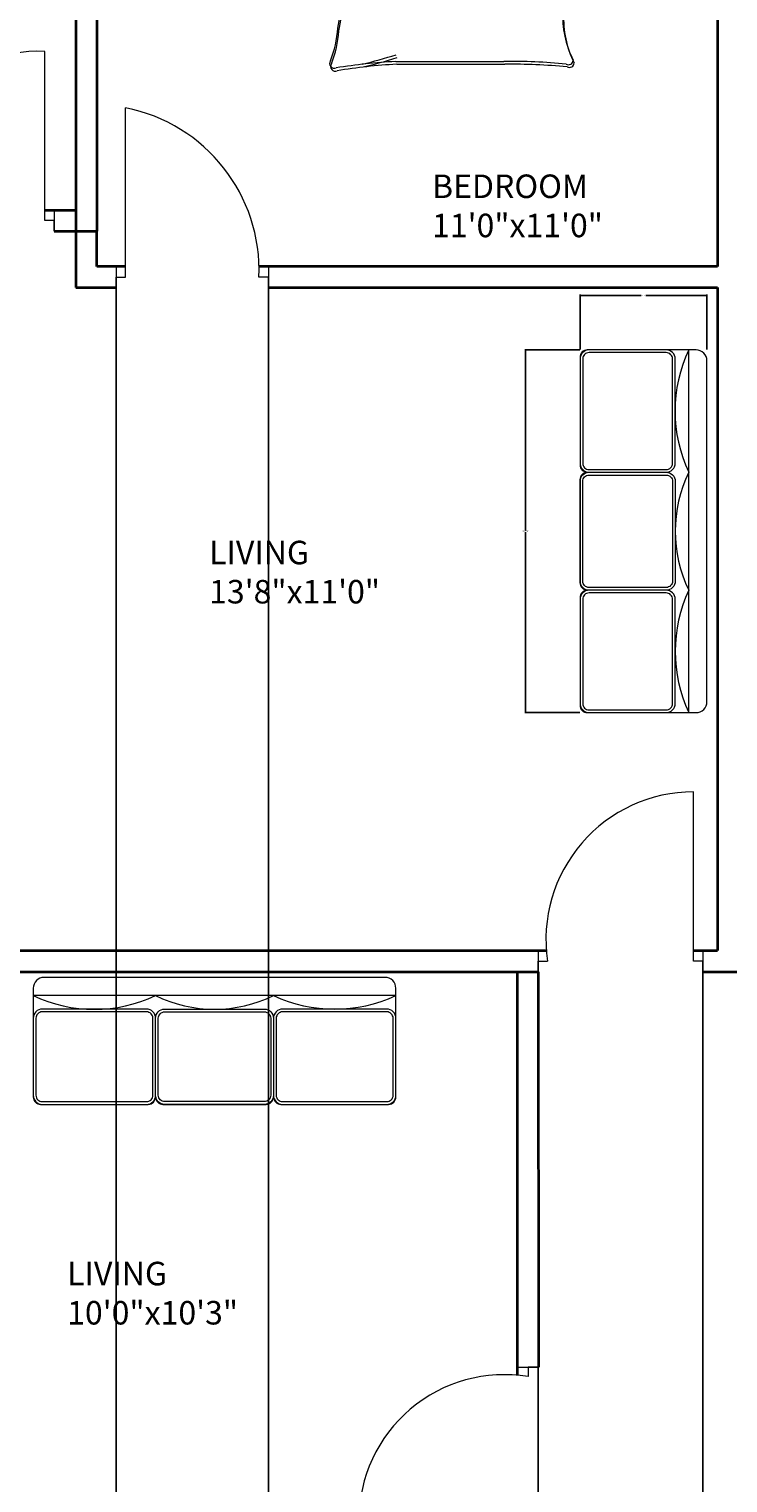
# Model space of a CAD drawing. Units: inches. Extents: x 2234 to 3001, y 1541 to 2386.
# Tile 6 of 12: x 2450 to 2599, y 1891 to 2201. Entities that reach past the tile are written whole.
import ezdxf

# ---------------------------------------------------------------- set-up
doc = ezdxf.new("R2010")
doc.units = ezdxf.units.IN
for name, color, linetype, lineweight in [('A-ANNO-DIMS', 2, 'Continuous', 18), ('A-AREA-IDEN', 7, 'Continuous', 18), ('A-DOOR', 3, 'Continuous', 18), ('A-FURN', 9, 'Continuous', 13), ('A-WALL', 7, 'Continuous', 35)]:
    doc.layers.add(name, color=color, linetype=linetype, lineweight=lineweight)
doc.styles.get("Standard").update_dxf_attribs({"font": 'arial.ttf'})
doc.dimstyles.get("Standard").update_dxf_attribs({"dimtxt": 0.18, "dimasz": 0.18, "dimexe": 0.18, "dimexo": 0.0625, "dimgap": 0.09, "dimtad": 0, "dimtih": 1, "dimtoh": 1, "dimdec": 4, "dimzin": 0, "dimdsep": 46, "dimtxsty": 'Standard', "dimcen": 0.09, "dimadec": 0, "dimazin": 0, "dimtfac": 1, "dimtdec": 4, "dimtofl": 0, "dimtmove": 0, "dimatfit": 3, "dimfxl": 1, "dimtolj": 1, "dimtzin": 0, "dimarcsym": 0})

# ---------------------------------------------------------------- blocks, each defined once
blk = doc.blocks.new('SOFA-3-SEAT')
for points in [[(1.93, 51.12), (18.33, 51.12, 0.414214), (20.26, 53.05), (20.26, 75.24, 0.414214), (18.33, 77.16), (1.93, 77.16, 0.414214), (0, 75.24), (0, 53.05, 0.414214)], [(1.93, 51.7), (18.33, 51.7, 0.414214), (19.68, 53.05), (19.68, 75.24, 0.414214), (18.33, 76.59), (1.93, 76.59, 0.414214), (0.58, 75.24), (0.58, 53.05, 0.414214)], [(1.93, 51.12), (18.33, 51.12, -0.414214), (20.26, 49.19), (20.26, 27.97, -0.414214), (18.33, 26.04), (1.93, 26.04, -0.414214), (0, 27.97), (0, 49.19, -0.414214)], [(1.93, 50.54), (18.33, 50.54, -0.414214), (19.68, 49.19), (19.68, 27.97, -0.414214), (18.33, 26.62), (1.93, 26.62, -0.414214), (0.58, 27.97), (0.58, 49.19, -0.414214)], [(1.93, 0), (18.33, 0, 0.414214), (20.26, 1.93), (20.26, 24.11, 0.414214), (18.33, 26.04), (1.93, 26.04, 0.414214), (0, 24.11), (0, 1.93, 0.414214)], [(1.93, 0.58), (18.33, 0.58, 0.414214), (19.68, 1.93), (19.68, 24.11, 0.414214), (18.33, 25.46), (1.93, 25.46, 0.414214), (0.58, 24.11), (0.58, 1.93, 0.414214)]]:
    blk.add_lwpolyline(points, format="xyb", close=True)
at = {"ltscale": 0.03}
blk.add_lwpolyline([(0, 24.48), (0, 1.54, 0.414214), (1.54, 0), (24.69, 0, 0.414214), (27.01, 2.31), (27.01, 74.85, 0.414214), (24.69, 77.16), (1.54, 77.16, 0.414214), (0, 75.62), (0, 52.68, 0.414214), (1.54, 51.14, -1), (1.54, 51.1, 0.414214), (0, 49.56), (0, 27.61, 0.414214), (1.54, 26.06, -1), (1.54, 26.02, 0.414214)], format="xyb", close=True, dxfattribs=at)
blk.add_lwpolyline([(23.15, 0), (23.15, 77.16)])
for centre, radius, start, end in [((50.64, 64.14), 30.42, 154.6538, 205.3462), ((48.71, 38.58), 28.47, 153.869, 206.131), ((50.96, 13.02), 30.71, 154.9106, 205.0894)]:
    blk.add_arc(centre, radius, start, end)
blk = doc.blocks.new('BED-DOUBLE-A')
for p, q in [((3.24, 59.14), (3.24, 76.05)), ((3.24, 59.14), (3.24, 76.05)), ((3.24, 74.62), (47.87, 74.62)), ((3.24, 74.62), (47.87, 74.62)), ((48.08, 76.05), (3.46, 76.05)), ((3.46, 58.54), (3.46, 75.45)), ((3.46, 58.54), (3.46, 75.45)), ((22.91, 73.76), (24.26, 74.3)), ((22.91, 73.76), (24.26, 74.3)), ((24.26, 74.3), (24.8, 69.31)), ((24.26, 74.3), (24.8, 69.31)), ((47.87, 76.05), (47.87, 51.2)), ((47.87, 76.05), (47.87, 51.2)), ((48.08, 76.05), (48.08, 75.45)), ((48.08, 75.45), (48.08, 50.6)), ((48.08, 75.45), (48.08, 50.6)), ((3.46, 74.02), (48.08, 74.02)), ((3.46, 74.02), (48.08, 74.02)), ((3.64, 72.93), (7.64, 73.24)), ((3.64, 72.93), (7.64, 73.24)), ((3.64, 72.95), (4.18, 69.98)), ((3.64, 72.95), (4.18, 69.98)), ((3.85, 72.33), (7.85, 72.64)), ((3.85, 72.33), (7.85, 72.64)), ((3.85, 72.35), (4.39, 69.38)), ((3.85, 72.35), (4.39, 69.38)), ((7.64, 73.24), (7.74, 73.22)), ((7.64, 73.24), (7.74, 73.22)), ((7.74, 73.22), (11.31, 72.95)), ((7.74, 73.22), (11.31, 72.95)), ((7.85, 72.64), (7.95, 72.62)), ((7.85, 72.64), (7.95, 72.62)), ((7.95, 72.62), (11.52, 72.35)), ((7.95, 72.62), (11.52, 72.35)), ((11.31, 72.95), (16.44, 72.01)), ((11.31, 72.95), (16.44, 72.01)), ((11.52, 72.35), (16.65, 71.41)), ((11.52, 72.35), (16.65, 71.41)), ((13.87, 72.55), (15.76, 73.22)), ((13.87, 72.55), (15.76, 73.22)), ((14.08, 71.95), (15.97, 72.62)), ((14.08, 71.95), (15.97, 72.62)), ((15.76, 73.22), (18.46, 73.9)), ((15.76, 73.22), (18.46, 73.9)), ((15.97, 72.62), (18.67, 73.3)), ((15.97, 72.62), (18.67, 73.3)), ((18.46, 73.9), (18.76, 73.9)), ((18.46, 73.9), (18.76, 73.9)), ((18.67, 73.3), (18.97, 73.3)), ((18.67, 73.3), (18.97, 73.3)), ((18.76, 73.9), (22.91, 73.76)), ((18.76, 73.9), (22.91, 73.76)), ((18.97, 73.3), (23.12, 73.16)), ((18.97, 73.3), (23.12, 73.16)), ((23.12, 73.16), (24.47, 73.7)), ((23.12, 73.16), (24.47, 73.7)), ((24.47, 73.7), (25.01, 68.71)), ((24.47, 73.7), (25.01, 68.71)), ((26.12, 73.72), (25.9, 68.7)), ((26.12, 73.72), (25.9, 68.7)), ((26.34, 73.12), (26.11, 68.1)), ((26.34, 73.12), (26.11, 68.1)), ((27.5, 73.27), (26.12, 73.72)), ((27.5, 73.27), (26.12, 73.72)), ((27.72, 72.67), (26.34, 73.12)), ((27.72, 72.67), (26.34, 73.12)), ((31.64, 73.66), (27.5, 73.27)), ((31.64, 73.66), (27.5, 73.27)), ((31.85, 73.06), (27.72, 72.67)), ((31.85, 73.06), (27.72, 72.67)), ((31.94, 73.68), (31.64, 73.66)), ((31.94, 73.68), (31.64, 73.66)), ((32.15, 73.08), (31.85, 73.06)), ((32.15, 73.08), (31.85, 73.06)), ((34.67, 73.17), (31.94, 73.68)), ((34.67, 73.17), (31.94, 73.68)), ((34.89, 72.58), (32.15, 73.08)), ((34.89, 72.58), (32.15, 73.08)), ((39.14, 73.18), (34.08, 71.92)), ((39.14, 73.18), (34.08, 71.92)), ((39.35, 72.58), (34.29, 71.32)), ((39.35, 72.58), (34.29, 71.32)), ((36.6, 72.62), (34.67, 73.17)), ((36.6, 72.62), (34.67, 73.17)), ((36.82, 72.02), (34.89, 72.58)), ((36.82, 72.02), (34.89, 72.58)), ((42.68, 73.67), (39.14, 73.18)), ((42.68, 73.67), (39.14, 73.18)), ((42.9, 73.08), (39.35, 72.58)), ((42.9, 73.08), (39.35, 72.58)), ((46.79, 73.66), (41.75, 73.75)), ((41.75, 73.75), (42.68, 73.67)), ((46.79, 73.66), (41.75, 73.75)), ((41.75, 73.75), (42.68, 73.67)), ((47.01, 73.06), (41.96, 73.15)), ((41.96, 73.15), (42.9, 73.08)), ((47, 73.06), (41.96, 73.15)), ((41.96, 73.15), (42.9, 73.08)), ((46.79, 73.66), (46.44, 70.66)), ((46.79, 73.66), (46.44, 70.66)), ((47.01, 73.06), (46.65, 70.07)), ((47, 73.06), (46.65, 70.07)), ((4.18, 69.98), (3.77, 67.55)), ((4.18, 69.98), (3.77, 67.55)), ((4.39, 69.38), (3.98, 66.95)), ((4.39, 69.38), (3.98, 66.95)), ((4.72, 67.69), (5.66, 70.25)), ((4.72, 67.69), (5.66, 70.25)), ((4.93, 67.09), (5.87, 69.65)), ((4.93, 67.09), (5.87, 69.65)), ((24.8, 69.31), (25.34, 66.34)), ((24.8, 69.31), (25.34, 66.34)), ((25.01, 68.71), (25.55, 65.74)), ((25.01, 68.71), (25.55, 65.74)), ((25.9, 68.7), (25.54, 65.7)), ((25.9, 68.7), (25.54, 65.7)), ((26.11, 68.1), (25.76, 65.11)), ((26.11, 68.1), (25.76, 65.11)), ((46.04, 68.34), (44.94, 70.84)), ((46.04, 68.34), (44.94, 70.84)), ((46.26, 67.74), (45.15, 70.24)), ((46.26, 67.74), (45.15, 70.24)), ((46.79, 65), (46.04, 68.34)), ((46.79, 65), (46.04, 68.34)), ((46.44, 70.66), (46.99, 68.26)), ((46.44, 70.66), (46.99, 68.26)), ((46.99, 68.26), (46.51, 67.28)), ((46.99, 68.26), (46.51, 67.28)), ((46.65, 70.07), (47.21, 67.66)), ((46.65, 70.07), (47.21, 67.66)), ((3.77, 67.55), (4.31, 66.61)), ((3.77, 67.55), (4.31, 66.61)), ((3.98, 66.95), (4.52, 66.01)), ((3.98, 66.95), (4.52, 66.01)), ((4.18, 64.31), (4.72, 67.69)), ((4.18, 64.31), (4.72, 67.69)), ((4.39, 63.71), (4.93, 67.09)), ((4.39, 63.71), (4.93, 67.09)), ((25.34, 65.12), (24.8, 63.37)), ((25.34, 65.12), (24.8, 63.37)), ((25.34, 66.34), (25.34, 65.12)), ((25.34, 66.34), (25.34, 65.12)), ((25.54, 65.7), (25.62, 64.49)), ((25.54, 65.7), (25.62, 64.49)), ((25.55, 65.74), (25.55, 64.52)), ((25.55, 65.74), (25.55, 64.52)), ((25.76, 65.11), (25.83, 63.89)), ((25.76, 65.11), (25.83, 63.89)), ((47.01, 64.41), (46.26, 67.74)), ((47, 64.41), (46.26, 67.74)), ((46.61, 63.5), (46.79, 65)), ((46.62, 63.5), (46.79, 65)), ((47.21, 67.66), (46.73, 66.69)), ((47.21, 67.66), (46.73, 66.69)), ((3.91, 59.86), (4.45, 62.83)), ((3.91, 59.86), (4.45, 62.83)), ((4.12, 59.26), (4.66, 62.23)), ((4.12, 59.26), (4.66, 62.23)), ((4.45, 62.83), (4.18, 64.31)), ((4.45, 62.83), (4.18, 64.31)), ((4.66, 62.23), (4.39, 63.71)), ((4.66, 62.23), (4.39, 63.71)), ((22.51, 60.86), (19.57, 61.88)), ((22.51, 60.86), (19.57, 61.88)), ((24.8, 63.37), (24.8, 60.86)), ((24.8, 63.37), (24.8, 60.86)), ((25.55, 64.52), (25.01, 62.77)), ((25.55, 64.52), (25.01, 62.77)), ((25.01, 62.77), (25.01, 60.27)), ((25.01, 62.77), (25.01, 60.27)), ((25.62, 64.49), (26.27, 62.77)), ((25.62, 64.49), (26.27, 62.77)), ((25.83, 63.89), (26.48, 62.18)), ((25.83, 63.89), (26.48, 62.18)), ((26.27, 62.77), (26.42, 60.27)), ((26.27, 62.77), (26.42, 60.27)), ((26.48, 62.18), (26.64, 59.68)), ((26.48, 62.18), (26.64, 59.68)), ((47.34, 60.57), (46.61, 63.5)), ((47.34, 60.57), (46.62, 63.5)), ((46.83, 62.91), (47.01, 64.41)), ((46.83, 62.91), (47, 64.41)), ((47.55, 59.98), (46.83, 62.91)), ((47.55, 59.98), (46.83, 62.91)), ((8.67, 60.53), (3.91, 59.86)), ((8.67, 60.53), (3.91, 59.86)), ((8.88, 59.93), (4.12, 59.26)), ((8.88, 59.93), (4.12, 59.26)), ((5.96, 61.45), (9.72, 60.83)), ((5.96, 61.45), (9.72, 60.83)), ((6.17, 60.86), (9.94, 60.24)), ((6.17, 60.86), (9.94, 60.24)), ((9.72, 60.83), (8.67, 60.53)), ((9.72, 60.83), (8.67, 60.53)), ((9.94, 60.24), (8.88, 59.93)), ((9.94, 60.24), (8.88, 59.93)), ((9.72, 60.83), (16.27, 60.43)), ((9.72, 60.83), (16.27, 60.43)), ((9.94, 60.24), (16.48, 59.83)), ((9.94, 60.24), (16.48, 59.83)), ((16.27, 60.43), (18.1, 60.95)), ((16.27, 60.43), (18.1, 60.95)), ((16.48, 59.83), (18.31, 60.35)), ((16.48, 59.83), (18.31, 60.35)), ((18.1, 60.95), (22.89, 60.57)), ((18.1, 60.95), (22.89, 60.57)), ((18.31, 60.35), (23.1, 59.98)), ((18.31, 60.35), (23.1, 59.98)), ((22.72, 60.27), (19.78, 61.28)), ((22.72, 60.27), (19.78, 61.28)), ((24.8, 60.86), (22.51, 60.86)), ((24.8, 60.86), (22.51, 60.86)), ((25.01, 60.27), (22.72, 60.27)), ((25.01, 60.27), (22.72, 60.27)), ((26.42, 60.27), (28.71, 60.42)), ((26.42, 60.27), (28.71, 60.42)), ((26.64, 59.68), (28.93, 59.82)), ((26.64, 59.68), (28.93, 59.82)), ((28.25, 59.82), (32.17, 53.75)), ((28.25, 59.82), (32.17, 53.75)), ((28.47, 59.22), (32.38, 53.16)), ((28.47, 59.22), (32.38, 53.16)), ((28.71, 60.42), (31.58, 61.62)), ((28.71, 60.42), (31.58, 61.62)), ((28.93, 59.82), (31.79, 61.02)), ((28.93, 59.82), (31.79, 61.02)), ((37.95, 57.08), (30.17, 59.82)), ((37.95, 57.08), (30.17, 59.82)), ((38.16, 56.48), (30.38, 59.22)), ((38.16, 56.48), (30.38, 59.22)), ((30.41, 61.45), (34.17, 60.83)), ((30.41, 61.45), (34.17, 60.83)), ((30.62, 60.86), (34.38, 60.24)), ((30.62, 60.86), (34.38, 60.24)), ((34.17, 60.83), (40.72, 60.43)), ((34.17, 60.83), (40.72, 60.43)), ((34.38, 60.24), (40.93, 59.83)), ((34.38, 60.24), (40.93, 59.83)), ((40.72, 60.43), (42.55, 60.95)), ((40.72, 60.43), (42.55, 60.95)), ((40.93, 59.83), (42.76, 60.35)), ((40.93, 59.83), (42.76, 60.35)), ((42.55, 60.95), (47.34, 60.57)), ((42.55, 60.95), (47.34, 60.57)), ((42.76, 60.35), (47.55, 59.98)), ((42.76, 60.35), (47.55, 59.98)), ((43.16, 55.2), (37.95, 57.08)), ((43.16, 55.2), (37.95, 57.08)), ((43.37, 54.6), (38.16, 56.48)), ((43.37, 54.6), (38.16, 56.48)), ((32.17, 53.75), (33.76, 49.56)), ((32.17, 53.75), (33.76, 49.56)), ((32.38, 53.16), (33.97, 48.97)), ((32.38, 53.16), (33.97, 48.97)), ((45.91, 53.18), (43.16, 55.2)), ((45.9, 53.18), (43.16, 55.2)), ((46.12, 52.58), (43.37, 54.6)), ((46.12, 52.58), (43.37, 54.6)), ((49.36, 50.14), (45.9, 53.18)), ((49.37, 50.14), (45.91, 53.18)), ((49.58, 49.54), (46.12, 52.58)), ((49.58, 49.54), (46.12, 52.58)), ((33.76, 49.56), (34.05, 47.68)), ((33.76, 49.56), (34.05, 47.68)), ((38.24, 49.13), (41.42, 49.56)), ((38.24, 49.13), (41.42, 49.56)), ((41.42, 49.56), (45.04, 49.85)), ((41.42, 49.56), (45.04, 49.85)), ((45.04, 49.85), (47.93, 49.56)), ((45.04, 49.85), (47.93, 49.56)), ((47.93, 49.56), (49.37, 50.14)), ((47.93, 49.56), (49.36, 50.14)), ((48.14, 48.97), (49.58, 49.54)), ((48.14, 48.97), (49.58, 49.54)), ((49.44, 48.51), (49.36, 50.14, 3.61)), ((49.44, 48.51), (49.37, 50.14, 3.61)), ((49.65, 47.91), (49.58, 49.54, 3.61)), ((49.65, 47.91), (49.58, 49.54, 3.61)), ((33.97, 48.97), (34.26, 47.09)), ((33.97, 48.97), (34.26, 47.09)), ((34.05, 47.68), (36.36, 48.26)), ((34.05, 47.68), (36.36, 48.26)), ((34.26, 47.09), (36.57, 47.66)), ((34.26, 47.09), (36.57, 47.66)), ((36.36, 48.26), (38.24, 49.13)), ((36.36, 48.26), (38.24, 49.13)), ((36.57, 47.66), (38.45, 48.53)), ((36.57, 47.66), (38.45, 48.53)), ((38.45, 48.53), (41.64, 48.97)), ((38.45, 48.53), (41.64, 48.97)), ((41.64, 48.97), (45.25, 49.25)), ((41.64, 48.97), (45.25, 49.25)), ((45.25, 49.25), (48.14, 48.97)), ((45.25, 49.25), (48.14, 48.97)), ((14.07, 2.05), (37.05, 2.05)), ((14.07, 2.05), (37.05, 2.05)), ((14.28, 1.46), (37.26, 1.46)), ((14.28, 1.46), (37.26, 1.46))]:
    blk.add_line(p, q)
for centre, radius, start, end in [((79.52, 57.28), 77.79, 178.7218, 185.604), ((79.52, 57.28), 77.79, 178.7218, 185.604), ((19.94, -93.94), 154.04, 86.0865, 96.7821), ((19.94, -93.94), 154.04, 86.0865, 96.7821), ((20.16, -94.54), 154.04, 86.0865, 96.7821), ((20.16, -94.54), 154.04, 86.0865, 96.7821), ((79.73, 56.69), 77.79, 178.7218, 185.604), ((79.73, 56.69), 77.79, 178.7218, 185.604), ((16.58, -69.91), 120.47, 81.7845, 96.9006), ((16.58, -69.91), 120.47, 81.7845, 96.9006), ((16.79, -70.51), 120.47, 81.7845, 96.9006), ((16.79, -70.51), 120.47, 81.7845, 96.9006), ((-156.22, 46.94), 158.84, 358.4762, 1.0082), ((-156.22, 46.94), 158.84, 358.4762, 1.0082), ((-156.01, 46.34), 158.84, 358.4762, 1.0082), ((-156.01, 46.34), 158.84, 358.4762, 1.0082), ((34.21, 47.63), 0.172, 160.2464, 271.1377), ((34.21, 47.63), 0.172, 160.2464, 271.1377), ((29.09, 74.66), 27.69, 280.6617, 289.8806), ((29.09, 74.66), 27.69, 280.6617, 289.8806), ((34.42, 47.03), 0.172, 160.2464, 271.1377), ((34.42, 47.03), 0.172, 160.2464, 271.1377), ((29.3, 74.07), 27.69, 280.6617, 289.8806), ((29.3, 74.07), 27.69, 280.6617, 289.8806), ((40.85, 43.3), 5.81, 78.6608, 113.7384), ((40.85, 43.3), 5.81, 78.6608, 113.7384), ((41.06, 42.71), 5.81, 78.6608, 113.7384), ((41.06, 42.71), 5.81, 78.6608, 113.7384), ((47.93, 82.26), 33.79, 259.8763, 272.5657), ((47.93, 82.26), 33.79, 259.8763, 272.5657), ((48.14, 81.67), 33.79, 259.8763, 272.5657), ((48.14, 81.67), 33.79, 259.8763, 272.5657), ((170.19, 42.14), 120.92, 176.9791, 183.8365), ((170.19, 42.14), 120.92, 176.9791, 183.8365), ((170.4, 41.54), 120.92, 176.9791, 183.8365), ((170.4, 41.54), 120.92, 176.9791, 183.8365), ((452.7, 28.79), 450.36, 178.2277, 181.7185), ((452.7, 28.79), 450.36, 178.2277, 181.7185), ((452.91, 28.19), 450.36, 178.2277, 181.7185), ((452.91, 28.19), 450.36, 178.2277, 181.7185), ((-4210.02, 12.72), 4259.62, 0.00217, 0.28689), ((-4210.02, 12.72), 4259.62, 0.00217, 0.28689), ((-4209.81, 12.12), 4259.62, 0.00217, 0.28689), ((-4209.81, 12.12), 4259.62, 0.00217, 0.28689), ((-25.12, 15.81), 27.67, 346.0648, 358.9113), ((-25.12, 15.81), 27.67, 346.0648, 358.9113), ((-24.9, 15.21), 27.67, 346.0648, 358.9113), ((-24.9, 15.21), 27.67, 346.0648, 358.9113), ((71.11, 11.93), 21.54, 177.4714, 206.4681), ((71.11, 11.93), 21.54, 177.4714, 206.4681), ((71.32, 11.33), 21.54, 177.4714, 206.4681), ((71.32, 11.33), 21.54, 177.4714, 206.4681), ((-20.22, 10.43), 22, 337.9751, 356.652), ((-20.22, 10.43), 22, 337.9751, 356.652), ((-20.01, 9.83), 22, 337.9751, 356.652), ((-20.01, 9.83), 22, 337.9751, 356.652), ((-16.08, 98.19), 99.41, 283.3832, 287.7053), ((-16.08, 98.19), 99.41, 283.3832, 287.7053), ((1.02, 1.61), 1.02, 146.1736, 293.4781), ((1.02, 1.61), 1.02, 146.1736, 293.4781), ((1.23, 1.01), 1.02, 146.1736, 293.4781), ((1.23, 1.01), 1.02, 146.1736, 293.4781), ((20.01, -111.48), 113.69, 92.9958, 99.4091), ((20.01, -111.48), 113.69, 92.9958, 99.4091), ((20.22, -112.08), 113.69, 92.9958, 99.4091), ((20.22, -112.08), 113.69, 92.9958, 99.4091), ((-15.87, 97.59), 99.41, 283.3832, 287.7053), ((-15.87, 97.59), 99.41, 283.3832, 287.7053), ((38.43, -122.16), 124.23, 84.4998, 90.6351), ((38.43, -122.16), 124.23, 84.4998, 90.6351), ((38.64, -122.76), 124.23, 84.4998, 90.6351), ((38.64, -122.76), 124.23, 84.4998, 90.6351), ((50.81, 2.4), 1.03, 242.6588, 356.02), ((50.8, 2.4), 1.03, 242.6588, 356.02), ((51.02, 1.81), 1.03, 242.6588, 356.02), ((51.02, 1.81), 1.03, 242.6588, 356.02)]:
    blk.add_arc(centre, radius, start, end)
blk = doc.blocks.new('*D21')
at = {"layer": 'A-ANNO-DIMS', "color": 0, "lineweight": -2, "transparency": 16777216}
for p, q in [((2567.47, 2132.38), (2555.78, 2132.38)), ((2555.96, 2132.2), (2555.96, 2093.98)), ((2555.96, 2055.4), (2555.96, 2093.61)), ((2567.47, 2055.22), (2555.78, 2055.22))]:
    blk.add_line(p, q, dxfattribs=at)
at = {"layer": 'A-ANNO-DIMS', "color": 0, "transparency": 16777216}
for points in [[(2555.93, 2132.2), (2555.99, 2132.2), (2555.96, 2132.38)], [(2555.93, 2055.4), (2555.99, 2055.4), (2555.96, 2055.22)]]:
    blk.add_solid(points, dxfattribs=at)
at = {"layer": 'Defpoints', "color": 0, "transparency": 16777216}
for p in [(2555.96, 2132.38), (2567.53, 2132.38), (2567.53, 2055.22)]:
    blk.add_point(p, dxfattribs=at)
at = {"layer": 'A-ANNO-DIMS', "color": 0, "transparency": 16777216, "insert": (2555.96, 2093.8), "char_height": 0.18, "attachment_point": 5}
blk.add_mtext('\\A1;SOFA 77 TYP.', dxfattribs=at)
blk = doc.blocks.new('*D22')
at = {"layer": 'A-ANNO-DIMS', "color": 0, "lineweight": -2, "transparency": 16777216}
for p, q in [((2567.53, 2132.44), (2567.53, 2144.13)), ((2567.71, 2143.95), (2580.51, 2143.95)), ((2594.36, 2143.95), (2581.57, 2143.95)), ((2594.54, 2132.44), (2594.54, 2144.13))]:
    blk.add_line(p, q, dxfattribs=at)
at = {"layer": 'A-ANNO-DIMS', "color": 0, "transparency": 16777216}
for points in [[(2567.71, 2143.98), (2567.71, 2143.92), (2567.53, 2143.95)], [(2594.36, 2143.98), (2594.36, 2143.92), (2594.54, 2143.95)]]:
    blk.add_solid(points, dxfattribs=at)
at = {"layer": 'Defpoints', "color": 0, "transparency": 16777216}
for p in [(2594.54, 2143.95), (2567.53, 2132.38), (2594.54, 2132.38)]:
    blk.add_point(p, dxfattribs=at)
at = {"layer": 'A-ANNO-DIMS', "color": 0, "transparency": 16777216, "insert": (2581.04, 2143.95), "char_height": 0.18, "attachment_point": 5}
blk.add_mtext('\\A1;27 TYP.', dxfattribs=at)
blk = doc.blocks.new('*D71')
at = {"layer": 'A-ANNO-DIMS', "color": 0, "lineweight": -2, "transparency": 16777216}
for p, q in [((2558.62, 2000.05), (2558.62, 1666.58)), ((2593.68, 2000.05), (2593.68, 1666.58)), ((2558.8, 1666.76), (2575.76, 1666.76)), ((2593.5, 1666.76), (2576.55, 1666.76))]:
    blk.add_line(p, q, dxfattribs=at)
at = {"layer": 'A-ANNO-DIMS', "color": 0, "transparency": 16777216}
for points in [[(2558.8, 1666.79), (2558.8, 1666.73), (2558.62, 1666.76)], [(2593.5, 1666.79), (2593.5, 1666.73), (2593.68, 1666.76)]]:
    blk.add_solid(points, dxfattribs=at)
at = {"layer": 'Defpoints', "color": 0, "transparency": 16777216}
for p in [(2558.62, 2000.11), (2593.68, 2000.11), (2593.68, 1666.76)]:
    blk.add_point(p, dxfattribs=at)
at = {"layer": 'A-ANNO-DIMS', "color": 0, "transparency": 16777216, "insert": (2576.15, 1666.76), "char_height": 0.18, "attachment_point": 5}
blk.add_mtext('\\A1;35.06', dxfattribs=at)
blk = doc.blocks.new('*D72')
at = {"layer": 'A-ANNO-DIMS', "color": 0, "lineweight": -2, "transparency": 16777216}
for p, q in [((2468.84, 2145.55), (2468.84, 1666.58)), ((2501.22, 2145.55), (2501.22, 1666.58)), ((2469.02, 1666.76), (2484.64, 1666.76)), ((2501.04, 1666.76), (2485.42, 1666.76))]:
    blk.add_line(p, q, dxfattribs=at)
at = {"layer": 'A-ANNO-DIMS', "color": 0, "transparency": 16777216}
for points in [[(2469.02, 1666.79), (2469.02, 1666.73), (2468.84, 1666.76)], [(2501.04, 1666.79), (2501.04, 1666.73), (2501.22, 1666.76)]]:
    blk.add_solid(points, dxfattribs=at)
at = {"layer": 'Defpoints', "color": 0, "transparency": 16777216}
for p in [(2468.84, 2145.61), (2501.22, 2145.61), (2501.22, 1666.76)]:
    blk.add_point(p, dxfattribs=at)
at = {"layer": 'A-ANNO-DIMS', "color": 0, "transparency": 16777216, "insert": (2485.03, 1666.76), "char_height": 0.18, "attachment_point": 5}
blk.add_mtext('\\A1;32.39', dxfattribs=at)

msp = doc.modelspace()

# ---------------------------------------------------------------- linework, layer by layer
at = {"layer": 'A-DOOR'}
for p, q in [((2453.6298, 2159.861), (2453.6298, 2195.861)), ((2470.8354, 2147.861), (2470.8354, 2183.861)), ((2455.6298, 2162.111), (2455.6298, 2157.611)), ((2455.6298, 2159.861), (2453.6298, 2159.861)), ((2455.6298, 2157.611), (2455.6298, 2159.861)), ((2468.8354, 2150.111), (2468.8354, 2145.611)), ((2501.2223, 2150.111), (2501.2223, 2145.611)), ((2468.8354, 2145.611), (2468.8354, 2147.861)), ((2468.8354, 2147.861), (2470.8354, 2147.861)), ((2501.2223, 2147.861), (2499.2223, 2147.861)), ((2501.2223, 2145.611), (2501.2223, 2147.861)), ((2591.6832, 2002.361), (2591.6832, 2038.361)), ((2558.623, 2004.611), (2558.623, 2000.111)), ((2593.6832, 2004.611), (2593.6832, 2000.111)), ((2558.623, 2000.111), (2558.623, 2002.361)), ((2558.623, 2002.361), (2560.623, 2002.361)), ((2593.6832, 2002.361), (2591.6832, 2002.361)), ((2593.6832, 2000.111), (2593.6832, 2002.361)), ((2554.2534, 1915.9636), (2558.7092, 1915.9682)), ((2558.7092, 1915.9682), (2556.4813, 1915.9659)), ((2556.4813, 1915.9659), (2556.4813, 1913.9659))]:
    msp.add_line(p, q, dxfattribs=at)
for centre, radius, start, end in [((2452.2624, 2167.5859), 28.3081, 87.231325, 195.836074), ((2464.048, 2149.3171), 35.2044, 357.62952, 78.883646), ((2591.6832, 2006.9619), 31.3992, 90, 188.425739), ((2551.4011, 1883.4842), 30.9021, 80.53786, 180)]:
    msp.add_arc(centre, radius, start, end, dxfattribs=at)
at = {"layer": 'A-WALL'}
for p, q in [((2464.7534, 2298.611), (2464.7534, 2157.611)), ((2460.2534, 2294.111), (2460.2534, 2162.111)), ((2596.7534, 2267.7185), (2596.7534, 2150.111)), ((2453.6298, 2162.111), (2460.2534, 2162.111)), ((2460.2534, 2162.111), (2460.2534, 2150.111)), ((2455.6298, 2157.611), (2464.7534, 2157.611)), ((2464.7534, 2150.111), (2464.7534, 2157.611)), ((2460.2534, 2150.111), (2460.2534, 2145.611)), ((2470.8354, 2150.111), (2464.7534, 2150.111)), ((2596.7534, 2150.111), (2499.2434, 2150.111)), ((2460.2534, 2145.611), (2468.8354, 2145.611)), ((2501.2223, 2145.611), (2596.7534, 2145.611)), ((2596.7534, 2145.611), (2596.7534, 2004.611)), ((2438.7534, 2004.611), (2560.3722, 2004.611)), ((2591.6832, 2004.611), (2596.7534, 2004.611)), ((2438.7534, 2000.111), (2558.623, 2000.111)), ((2554.2534, 1914.2545), (2554.2534, 2000.111)), ((2558.623, 2000.111), (2558.7092, 1915.9682)), ((2593.6832, 2000.111), (2605.0604, 2000.111))]:
    msp.add_line(p, q, dxfattribs=at)

# ---------------------------------------------------------------- block references
at = {"layer": 'A-FURN'}
for name, p in [('BED-DOUBLE-A', (2514.2466, 2191.6708)), ('SOFA-3-SEAT', (2567.534, 2055.216))]:
    msp.add_blockref(name, p, dxfattribs=at)
at = {"layer": 'A-FURN', "rotation": 90}
msp.add_blockref('SOFA-3-SEAT', (2528.353, 1971.8828), dxfattribs=at)
msp.add_blockref('SOFA-3-SEAT', (2528.353, 1971.8828), dxfattribs=at)

# ---------------------------------------------------------------- texts
at = {"layer": 'A-AREA-IDEN', "char_height": 5, "attachment_point": 1}
for s, width, insert in [('BEDROOM\\P11\'0"x11\'0"', 86.749821, (2536.0428, 2169.6747)), ('LIVING\\P13\'8"x11\'0"', 161.186075, (2488.6147, 2091.772)), ('LIVING\\P10\'0"x10\'3"', 88.128412, (2458.4102, 1938.3946))]:
    msp.add_mtext_dynamic_manual_height_columns(s, width=width, gutter_width=12.5, heights=[0], dxfattribs=dict(at, insert=insert))

# ---------------------------------------------------------------- dimensions: what is measured, and where the dimension line sits
at = {"layer": 'A-ANNO-DIMS'}
for base, p1, p2, picture, middle in [((2501.2223, 1666.761), (2468.8354, 2145.611), (2501.2223, 2145.611), '*D72', (2485.0289, 1666.761)), ((2593.6832, 1666.761), (2558.623, 2000.111), (2593.6832, 2000.111), '*D71', (2576.1531, 1666.761))]:
    dim = msp.add_linear_dim(base=base, p1=p1, p2=p2, dimstyle='Standard', override={"dimdec": 2, "dimlfac": 1, "dimrnd": 0, "dimzin": 0, "dimdsep": 46, "dimlunit": 2}, dxfattribs=at)
    dim.commit()
    dim.dimension.update_dxf_attribs({"geometry": picture, "text_midpoint": middle})
dim = msp.add_linear_dim(base=(2594.5416, 2143.9549), p1=(2567.5341, 2132.3802), p2=(2594.5416, 2132.3802), text='<> TYP.', dimstyle='Standard', override={"dimdec": 0, "dimlfac": 1, "dimrnd": 0, "dimzin": 0, "dimdsep": 46, "dimlunit": 2}, dxfattribs=at)
dim.commit()
dim.dimension.update_dxf_attribs({"geometry": '*D22', "text_midpoint": (2581.0378, 2143.9549)})
dim = msp.add_linear_dim(base=(2555.9594, 2132.3802), p1=(2567.5341, 2055.2158), p2=(2567.5341, 2132.3802), angle=90, text='SOFA <> TYP.', dimstyle='Standard', override={"dimdec": 0, "dimlfac": 1, "dimrnd": 0, "dimzin": 0, "dimdsep": 46, "dimlunit": 2}, dxfattribs=at)
dim.commit()
dim.dimension.update_dxf_attribs({"geometry": '*D21', "text_midpoint": (2555.9594, 2093.798)})

doc.saveas('drawing.dxf')
